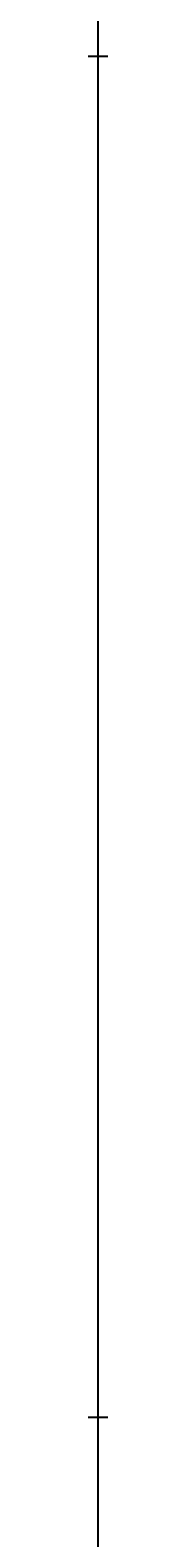
# Model space of a CAD drawing. Units: inches. Extents: x 35362 to 73946, y 43607 to 67532.
# Tile 39 of 134: x 48373 to 48373, y 46091 to 46564. Entities that reach past the tile are written whole.
import ezdxf

# ---------------------------------------------------------------- set-up
doc = ezdxf.new("R2010")
doc.units = ezdxf.units.IN
doc.header["$MEASUREMENT"] = 0
doc.layers.add('A-ANNO-DIMS', color=2, linetype='Continuous', lineweight=18)
doc.styles.get("Standard").update_dxf_attribs({"font": 'arial.ttf'})
doc.dimstyles.get("Standard").update_dxf_attribs({"dimtxt": 0.18, "dimasz": 0.18, "dimexe": 0.18, "dimexo": 0.0625, "dimgap": 0.09, "dimtad": 0, "dimtih": 1, "dimtoh": 1, "dimdec": 4, "dimzin": 0, "dimdsep": 46, "dimtxsty": 'Standard', "dimcen": 0.09, "dimadec": 0, "dimazin": 0, "dimtfac": 1, "dimtdec": 4, "dimtofl": 0, "dimtmove": 0, "dimatfit": 3, "dimfxl": 1, "dimtolj": 1, "dimtzin": 0, "dimarcsym": 0})

# ---------------------------------------------------------------- blocks, each defined once
blk = doc.blocks.new('*D5')
at = {"layer": 'A-ANNO-DIMS', "color": 0, "lineweight": -2, "transparency": 16777216}
for p, q in [((37121.95, 46919.32), (37121.95, 43606.68)), ((69871.5, 45449.83), (69871.5, 43606.68)), ((37122.13, 43606.86), (53496.29, 43606.86)), ((69871.32, 43606.86), (53497.15, 43606.86))]:
    blk.add_line(p, q, dxfattribs=at)
at = {"layer": 'A-ANNO-DIMS', "color": 0, "transparency": 16777216}
for points in [[(37122.13, 43606.89), (37122.13, 43606.83), (37121.95, 43606.86)], [(69871.32, 43606.89), (69871.32, 43606.83), (69871.5, 43606.86)]]:
    blk.add_solid(points, dxfattribs=at)
at = {"layer": 'Defpoints', "color": 0, "transparency": 16777216}
for p in [(37121.95, 46919.38), (69871.5, 45449.89), (69871.5, 43606.86)]:
    blk.add_point(p, dxfattribs=at)
at = {"layer": 'A-ANNO-DIMS', "color": 0, "transparency": 16777216, "insert": (53496.72, 43606.86), "char_height": 0.18, "attachment_point": 5}
blk.add_mtext('\\A1;32750', dxfattribs=at)
blk = doc.blocks.new('*D11')
at = {"layer": 'A-ANNO-DIMS', "color": 0, "lineweight": -2, "transparency": 16777216}
for p, q in [((47978.66, 56028.77), (47978.66, 43606.68)), ((53109.76, 56028.77), (53109.76, 43606.68)), ((47978.84, 43606.86), (50543.87, 43606.86)), ((53109.58, 43606.86), (50544.55, 43606.86))]:
    blk.add_line(p, q, dxfattribs=at)
at = {"layer": 'A-ANNO-DIMS', "color": 0, "transparency": 16777216}
for points in [[(47978.84, 43606.89), (47978.84, 43606.83), (47978.66, 43606.86)], [(53109.58, 43606.89), (53109.58, 43606.83), (53109.76, 43606.86)]]:
    blk.add_solid(points, dxfattribs=at)
at = {"layer": 'Defpoints', "color": 0, "transparency": 16777216}
for p in [(47978.66, 56028.84), (53109.76, 56028.84), (53109.76, 43606.86)]:
    blk.add_point(p, dxfattribs=at)
at = {"layer": 'A-ANNO-DIMS', "color": 0, "transparency": 16777216, "insert": (50544.21, 43606.86), "char_height": 0.18, "attachment_point": 5}
blk.add_mtext('\\A1;5131', dxfattribs=at)
blk = doc.blocks.new('*D13')
at = {"layer": 'A-ANNO-DIMS', "color": 0, "lineweight": -2, "transparency": 16777216}
for p, q in [((48373.49, 51694.02), (48373.49, 43606.68)), ((51029.04, 51694.02), (51029.04, 43606.68)), ((48373.67, 43606.86), (49700.8, 43606.86)), ((51028.86, 43606.86), (49701.73, 43606.86))]:
    blk.add_line(p, q, dxfattribs=at)
at = {"layer": 'A-ANNO-DIMS', "color": 0, "transparency": 16777216}
for points in [[(48373.67, 43606.89), (48373.67, 43606.83), (48373.49, 43606.86)], [(51028.86, 43606.89), (51028.86, 43606.83), (51029.04, 43606.86)]]:
    blk.add_solid(points, dxfattribs=at)
at = {"layer": 'Defpoints', "color": 0, "transparency": 16777216}
for p in [(48373.49, 51694.09), (51029.04, 51694.09), (51029.04, 43606.86)]:
    blk.add_point(p, dxfattribs=at)
at = {"layer": 'A-ANNO-DIMS', "color": 0, "transparency": 16777216, "insert": (49701.27, 43606.86), "char_height": 0.18, "attachment_point": 5}
blk.add_mtext('\\A1;2655.6', dxfattribs=at)
blk = doc.blocks.new('*D67')
at = {"layer": 'A-ANNO-DIMS', "color": 0, "lineweight": -2, "transparency": 16777216}
for p, q in [((56873.54, 53351.53), (35361.77, 53351.53)), ((35361.95, 53351.35), (35361.95, 49400.89)), ((35361.95, 45450.07), (35361.95, 49400.53)), ((53793.58, 45449.89), (35361.77, 45449.89))]:
    blk.add_line(p, q, dxfattribs=at)
at = {"layer": 'A-ANNO-DIMS', "color": 0, "transparency": 16777216}
for points in [[(35361.92, 53351.35), (35361.98, 53351.35), (35361.95, 53351.53)], [(35361.92, 45450.07), (35361.98, 45450.07), (35361.95, 45449.89)]]:
    blk.add_solid(points, dxfattribs=at)
at = {"layer": 'Defpoints', "color": 0, "transparency": 16777216}
for p in [(35361.95, 53351.53), (56873.6, 53351.53), (53793.64, 45449.89)]:
    blk.add_point(p, dxfattribs=at)
at = {"layer": 'A-ANNO-DIMS', "color": 0, "transparency": 16777216, "insert": (35361.95, 49400.71), "char_height": 0.18, "attachment_point": 5}
blk.add_mtext('\\A1;7901.6', dxfattribs=at)
blk = doc.blocks.new('*D76')
at = {"layer": 'A-ANNO-DIMS', "color": 0, "lineweight": -2, "transparency": 16777216}
for p, q in [((54052.84, 46555.29), (35361.77, 46555.29)), ((35361.95, 46555.11), (35361.95, 46342.27)), ((35361.95, 46129.06), (35361.95, 46341.9)), ((53793.58, 46128.88), (35361.77, 46128.88))]:
    blk.add_line(p, q, dxfattribs=at)
at = {"layer": 'A-ANNO-DIMS', "color": 0, "transparency": 16777216}
for points in [[(35361.92, 46555.11), (35361.98, 46555.11), (35361.95, 46555.29)], [(35361.92, 46129.06), (35361.98, 46129.06), (35361.95, 46128.88)]]:
    blk.add_solid(points, dxfattribs=at)
at = {"layer": 'Defpoints', "color": 0, "transparency": 16777216}
for p in [(35361.95, 46555.29), (54052.9, 46555.29), (53793.64, 46128.88)]:
    blk.add_point(p, dxfattribs=at)
at = {"layer": 'A-ANNO-DIMS', "color": 0, "transparency": 16777216, "insert": (35361.95, 46342.09), "char_height": 0.18, "attachment_point": 5}
blk.add_mtext('\\A1;426.4', dxfattribs=at)
blk = doc.blocks.new('*D90')
at = {"layer": 'A-ANNO-DIMS', "color": 0, "lineweight": -2, "transparency": 16777216}
for p, q in [((53707.72, 47291.29), (35361.77, 47291.29)), ((35361.95, 47291.11), (35361.95, 46710.26)), ((35361.95, 46129.06), (35361.95, 46709.9)), ((53793.58, 46128.88), (35361.77, 46128.88))]:
    blk.add_line(p, q, dxfattribs=at)
at = {"layer": 'A-ANNO-DIMS', "color": 0, "transparency": 16777216}
for points in [[(35361.92, 47291.11), (35361.98, 47291.11), (35361.95, 47291.29)], [(35361.92, 46129.06), (35361.98, 46129.06), (35361.95, 46128.88)]]:
    blk.add_solid(points, dxfattribs=at)
at = {"layer": 'Defpoints', "color": 0, "transparency": 16777216}
for p in [(53707.78, 47291.29), (35361.95, 46128.88), (53793.64, 46128.88)]:
    blk.add_point(p, dxfattribs=at)
at = {"layer": 'A-ANNO-DIMS', "color": 0, "transparency": 16777216, "insert": (35361.95, 46710.08), "char_height": 0.18, "attachment_point": 5}
blk.add_mtext('\\A1;1162.4', dxfattribs=at)

msp = doc.modelspace()

# ---------------------------------------------------------------- dimensions: what is measured, and where the dimension line sits
at = {"layer": 'A-ANNO-DIMS'}
for base, p1, p2, override, picture, middle in [((53109.76, 43606.859), (47978.665, 56028.836), (53109.76, 56028.836), {"dimdec": 0, "dimlfac": 1, "dimrnd": 0, "dimzin": 0, "dimdsep": 46, "dimlunit": 2}, '*D11', (50544.212, 43606.859)), ((51029.043, 43606.859), (48373.492, 51694.087), (51029.043, 51694.087), {"dimdec": 1, "dimlfac": 1, "dimrnd": 0, "dimzin": 0, "dimdsep": 46, "dimlunit": 2}, '*D13', (49701.267, 43606.859)), ((69871.496, 43606.859), (37121.949, 46919.381), (69871.496, 45449.894), {"dimdec": 0, "dimlfac": 1, "dimrnd": 0, "dimzin": 0, "dimdsep": 46, "dimlunit": 2}, '*D5', (53496.723, 43606.859))]:
    dim = msp.add_linear_dim(base=base, p1=p1, p2=p2, dimstyle='Standard', override=override, dxfattribs=at)
    dim.commit()
    dim.dimension.update_dxf_attribs({"geometry": picture, "text_midpoint": middle})
for base, p1, p2, picture, middle in [((35361.949, 53351.529), (53793.638, 45449.894), (56873.602, 53351.529), '*D67', (35361.949, 49400.712)), ((35361.949, 46128.878), (53707.781, 47291.285), (53793.638, 46128.878), '*D90', (35361.949, 46710.081)), ((35361.949, 46555.293), (53793.638, 46128.878), (54052.899, 46555.293), '*D76', (35361.949, 46342.086))]:
    dim = msp.add_linear_dim(base=base, p1=p1, p2=p2, angle=90, dimstyle='Standard', override={"dimdec": 1, "dimlfac": 1, "dimrnd": 0, "dimzin": 0, "dimdsep": 46, "dimlunit": 2}, dxfattribs=at)
    dim.commit()
    dim.dimension.update_dxf_attribs({"geometry": picture, "text_midpoint": middle})

doc.saveas('drawing.dxf')
